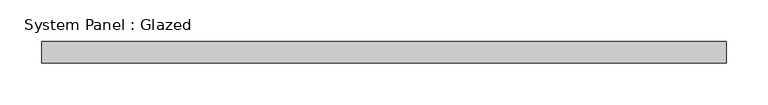
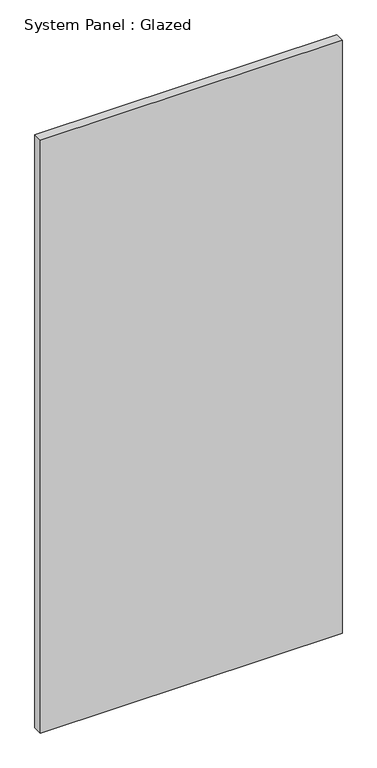
"""IFC4 building model written with IfcOpenShell, lengths in millimetres: plate geometry, System Panel : Glazed."""

from ifc_helpers import new_model, si_unit, origin, origin_with_axes, place, context, project, spatial, polyline, outline, extrude, source, transform, mapped, element, save


def system_panel_glazed_0f3f94b3(model_context):
    return source(origin(), model_context, "Body", "SweptSolid", [
        extrude(outline(polyline([(409.575, 19.05), (-409.575, 19.05), (-409.575, 44.45), (409.575, 44.45), (409.575, 19.05)])), origin_with_axes(), (0.0, 0.0, 1.0), 1701.8),
    ])


if __name__ == "__main__":
    model = new_model("IFC4")
    model_context = context("Model", 3, world=origin())
    ifc_project = project(units=[si_unit("LENGTHUNIT", "METRE", prefix="MILLI")], contexts=[model_context])
    site = spatial("IfcSite", under=ifc_project)
    building = spatial("IfcBuilding", under=site)
    placement = place(None, origin())
    system_panel_glazed_shape = system_panel_glazed_0f3f94b3(model_context)
    element("IfcPlate", 1, ObjectType="System Panel : Glazed", at=placement, inside=building, context=model_context, shape_type="MappedRepresentation", body=[
        mapped(system_panel_glazed_shape, transform((0.0, 0.0, 0.0), x_axis=(1.0, 0.0, 0.0), y_axis=(0.0, 1.0, 0.0), z_axis=(0.0, 0.0, 1.0))),
    ])
    save(model, "model.ifc")

# Revit data of these elements
# Type "System Panel : Glazed"
#   Construction Type Id = "GSP4R"
#   Analytic Construction = "1/8 in Pilkington single glazing"
#   Visual Light Transmittance = 0.9
#   Solar Heat Gain Coefficient = 0.86
#   Heat Transfer Coefficient (U) = 1.18115 BTU/(h·ft²·°F)
#   Define Thermal Properties by = 1
# Element 1 (IfcPlate, "System Panel : Glazed")
#   Materials on its faces: "Glass"
# Materials
#   "Glass": class "Glass", colour RGB 0 128 192, transparency 0.75, Description = "Soda Lime Glass", Cost = 0
